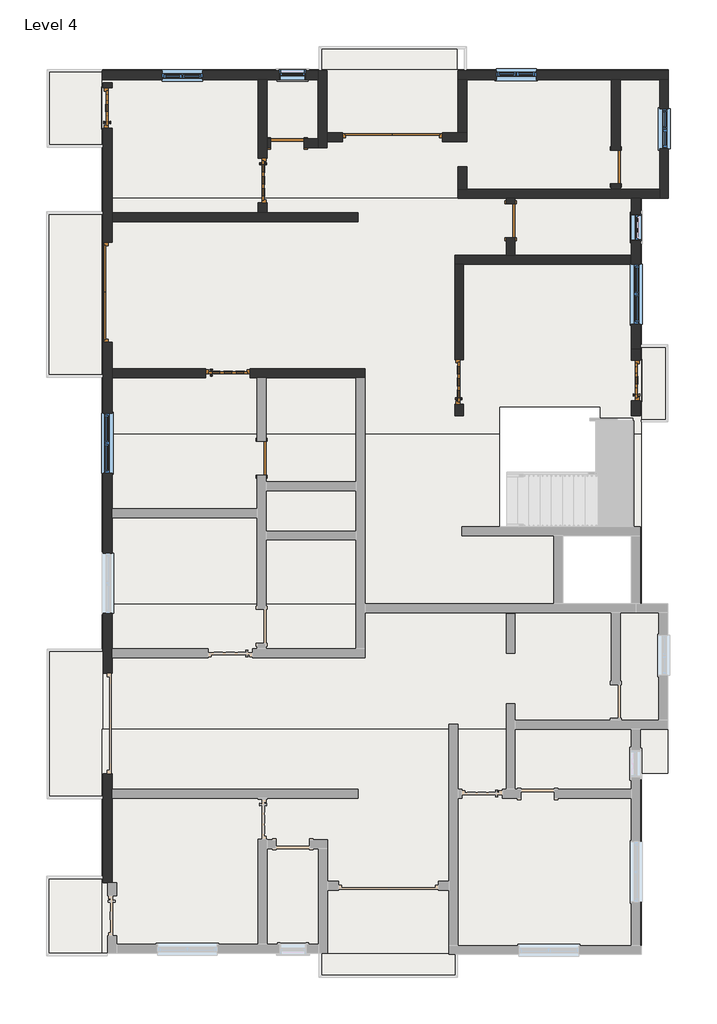
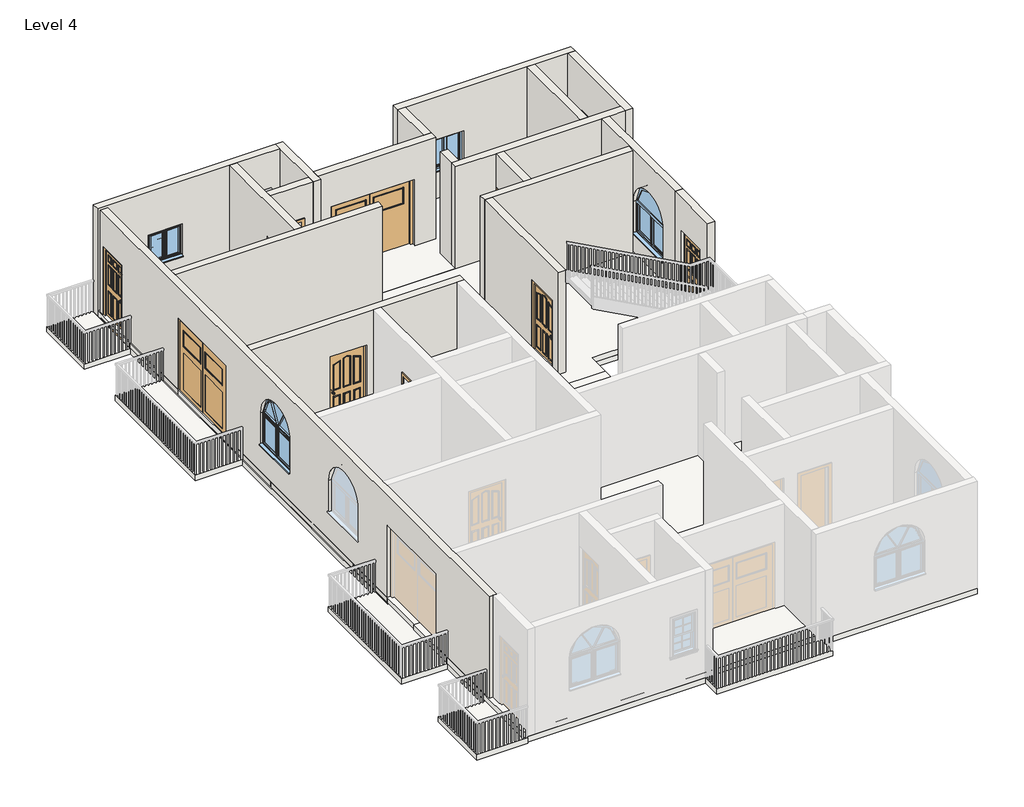
# One storey, part 2 of 7: 19 walls, 11 doors, 10 slabs, 7 windows, 5 roofs.
# Revit data of these elements (continued)
# Type "Windows_Dbl_w-Glazing_Bars : 910x910mm" (continued)
#   Window Board Extension = 0' - 0.98425"
#   Visual Light Transmittance = 0.9
#   Solar Heat Gain Coefficient = 0.78
#   Rough Width = 2' - 11.82677"
#   Rough Height = 2' - 11.82677"
#   Height = 2' - 11.82677"
#   Width = 2' - 11.82677"
#   Heat Transfer Coefficient (U) = 0.6496 BTU/(h·ft²·°F)
#   Glazing Thickness = 0' - 0.94488"
#   Glazing Bar Thickness = 0' - 0.7874"
#   FrameOffset - External = 0' - 1.9685"
#   Frame Depth = 0' - 2.55906"
#   Default Head Height = 6' - 10.67717"
#   Cill Depth = 0' - 3.44488"
#   Cavity Closer Width = 0' - 1.9685"
#   Cavity Closer Offset from Ext = 0' - 4.03543"
#   Cavity Closer Depth = 0' - 3.34646"
#   Vis - Glazing Bars = yes
#   Vis - Cavity Closers = yes
#   Define Thermal Properties by = 1
#   Material Trim = Window Frame
#   Material Glazing Bars = Window Frame
#   Material Glass = Glass
#   Material Frame = Window Frame
#   Wall Closure = (empty or 0)
# Elements 1, 2 (IfcDoor, "Doors_ExtSgl_5 : 910x2110mm")
#   Phase Created = New Construction
#   Materials on its faces: "Door - Panel", "Door - Handle", "Door - Frame/Mullion", "Door - Glazing"
# Elements 3, 4, 5 (IfcDoor, "Doors_ExtSgl_6 : 1010x2110mm")
#   Phase Created = New Construction
#   Materials on its faces: "Door - Panel", "Door - Handle", "Door - Frame/Mullion", "Door - Glazing"
# Element 6 (IfcDoor, "Doors_Garage_Timber_Side_Hung_Glazing : 2270x2050mm")
#   Phase Created = New Construction
#   Materials on its faces: "Door - Panel", "Door - Frame/Mullion", "Door - Glazing"
# Element 7 (IfcDoor, "Doors_Garage_Timber_Side_Hung_Glazing : 2270x2200mm")
#   Phase Created = New Construction
#   Materials on its faces: "Door - Panel", "Door - Frame/Mullion", "Door - Glazing"
# Elements 8, 9, 10, 11 (IfcDoor, "Single-Flush : 30\" x 80\"")
#   Phase Created = New Construction
#   Materials on its faces: "Door - Frame", "Door - Panel"
# Elements 12, 16 (IfcRoof, "Generic - 12\"")
#   built-in parameter 1001705 = 30.5 (stored number, unit not read)
#   built-in parameter 1001710 = 33615
#   Phase Created = New Construction
#   Materials on its faces: "Default Roof", "Earth"
# Elements 13, 15 (IfcRoof, "Generic - 12\"")
#   built-in parameter 1001705 = 30.5 (stored number, unit not read)
#   built-in parameter 1001710 = 33615
#   Phase Created = New Construction
#   Materials on its faces: "Default Roof", "Wood - Stained"
# Element 14 (IfcRoof, "Generic - 12\"")
#   built-in parameter 1001705 = 30.5 (stored number, unit not read)
#   built-in parameter 1001710 = 33615
#   Phase Created = New Construction
#   Materials on its faces: "Default Roof", "Concrete, Lightweight"
# Element 17 (IfcSlab, "Generic - 12\"")
#   Height Offset From Level = 0' - 0"
#   Phase Created = New Construction
#   Materials on its faces: "Default Floor", "Concrete, Lightweight"
# Element 18 (IfcSlab, "Generic - 12\"")
#   Height Offset From Level = 0' - 0"
#   Phase Created = New Construction
#   Materials on its faces: "Default Floor", "Concrete, Lightweight", "Wood - Stained", "Earth"
# Element 19 (IfcSlab, "Generic - 12\"")
#   Height Offset From Level = 0' - 0"
#   Phase Created = New Construction
#   Materials on its faces: "Default Floor", "Earth"
# Element 20 (IfcSlab, "Generic - 12\"")
#   Height Offset From Level = 0' - 0"
#   Phase Created = New Construction
#   Materials on its faces: "Default Floor", "Brick, Soldier Course"
# Elements 21, 22, 23, 24, 25 (IfcSlab, "Generic - 12\"")
#   Height Offset From Level = 0' - 0"
#   Phase Created = New Construction
#   Materials on its faces: "Default Floor"
# Element 26 (IfcSlab, "Generic - 12\"")
#   Height Offset From Level = 0' - 0"
#   Phase Created = New Construction
#   Materials on its faces: "Default Floor", "Earth", "Concrete, Lightweight"
# Elements 27, 31 (IfcWall, "Generic - 9\" w")
#   Top Offset = 0' - 0"
#   Base Offset = 0' - 0"
#   wall height = 10' - 0"
#   Phase Created = New Construction
#   Base Constraint = Level 4
#   Top Constraint = Level 5
#   Materials on its faces: "Default Wall", "Earth"
# Element 28 (IfcWall, "Generic - 9\" w")
#   Top Offset = 0' - 0"
#   Base Offset = 0' - 0"
#   wall height = 10' - 0"
#   Phase Created = New Construction
#   Base Constraint = Level 4
#   Top Constraint = Level 5
#   Materials on its faces: "Default Wall", "Wood - Stained"
# Element 29 (IfcWall, "Generic - 9\" w")
#   Top Offset = 0' - 0"
#   Base Offset = 0' - 0"
#   wall height = 10' - 0"
#   Phase Created = New Construction
#   Base Constraint = Level 4
#   Top Constraint = Level 5
#   Materials on its faces: "Default Wall", "Grass"
# Element 30 (IfcWall, "Generic - 9\" w")
#   Top Offset = 0' - 0"
#   Base Offset = 0' - 0"
#   wall height = 10' - 0"
#   Phase Created = New Construction
#   Base Constraint = Level 4
#   Top Constraint = Level 5
#   Materials on its faces: "Default Wall", "mm"
# Elements 32, 33, 35, 37, 38, 40, 41, 42, 43, 44, 45 (IfcWall, "Generic -4.5\" p")
#   Top Offset = 0' - 0"
#   Base Offset = 0' - 0"
#   wall height = 10' - 0"
#   Phase Created = New Construction
#   Base Constraint = Level 4
#   Top Constraint = Level 5
#   Materials on its faces: "Default Wall"
# Elements 34, 39 (IfcWall, "Generic -4.5\" p")
#   Top Offset = 0' - 0"
#   Base Offset = 0' - 0"
#   wall height = 10' - 0"
#   Phase Created = New Construction
#   Base Constraint = Level 4
#   Top Constraint = Level 5
#   Materials on its faces: "Default Wall", "Earth"
# Element 36 (IfcWall, "Generic -4.5\" p")
#   Top Offset = 0' - 0"
#   Base Offset = 0' - 0"
#   wall height = 10' - 0"
#   Phase Created = New Construction
#   Base Constraint = Level 4
#   Top Constraint = Level 5
#   Materials on its faces: "Default Wall", "Oak Flooring"
# Element 46 (IfcWindow, "Window-Double-Hung : 24\" x 42\"")
#   Mark = "48"
#   Window Inset = 0' - 0"
#   Interior Wall Closure = 0' - 1 1/2"
#   Frame Extension = 0' - 1 1/4"
#   Exterior Wall Closure = 0' - 0 1/2"
#   Interior Trim Visibility = yes
#   Indicator Visibility = yes
#   Exterior Trim Visibility = yes
#   Phase Created = New Construction
#   Materials on its faces: "Wood - Stained", "Glass", "Clad - White"
# Element 47 (IfcWindow, "Window-Double-Hung : 24\" x 42\"")
#   Mark = "54"
#   Window Inset = 0' - 0"
#   Interior Wall Closure = 0' - 1 1/2"
#   Frame Extension = 0' - 1 1/4"
#   Exterior Wall Closure = 0' - 0 1/2"
#   Interior Trim Visibility = yes
#   Indicator Visibility = yes
#   Exterior Trim Visibility = yes
#   Phase Created = New Construction
#   Materials on its faces: "Wood - Stained", "Glass", "Clad - White"
# Element 48 (IfcWindow, "Windows_Arched : 1360x910mm")
#   Mark = "44"
#   Phase Created = New Construction
#   Materials on its faces: "Window Frame", "Glass"
# Element 49 (IfcWindow, "Windows_Arched : 1360x910mm")
#   Mark = "55"
#   Phase Created = New Construction
#   Materials on its faces: "Window Frame", "Glass"
# Element 50 (IfcWindow, "Windows_Dbl_w-Glazing_Bars : 910x910mm")
#   Mark = "51"
#   Phase Created = New Construction
#   Materials on its faces: "Window Frame", "Glass"
# Element 51 (IfcWindow, "Windows_Dbl_w-Glazing_Bars : 910x910mm")
#   Mark = "52"
#   Phase Created = New Construction
#   Materials on its faces: "Window Frame", "Glass"
# Element 52 (IfcWindow, "Windows_Dbl_w-Glazing_Bars : 910x910mm")
#   Mark = "53"
#   Phase Created = New Construction
#   Materials on its faces: "Window Frame", "Glass"
# Materials
#   "Door - Glazing": colour RGB 0 0 255, transparency 0.75
#   "Door - Panel": class "Wood", colour RGB 210 159 95, transparency 0, Cost = 0
#   "Door - Frame/Mullion": class "Wood", colour RGB 212 179 113, transparency 0
#   "Door - Handle": colour RGB 0 0 0, transparency 0
#   "Door - Frame": colour RGB 118 70 51, transparency 0, Cost = 0
#   "Wood - Stained": class "Wood", colour RGB 224 178 126, transparency 0, Cost = 0
#   "Clad - White": class "Wood", colour RGB 242 242 238, transparency 0, Cost = 0
#   "Glass": class "Glass", colour RGB 0 128 192, transparency 0.75, Description = "Soda Lime Glass", Cost = 0
#   "Window Frame": colour RGB 249 249 249, transparency 0
#   "Default Roof": colour RGB 88 101 114, transparency 0, Cost = 0
#   "Earth": class "Generic", colour RGB 97 75 62, transparency 0, Description = "Soil", Cost = 0
#   "Concrete, Lightweight": class "Concrete", colour RGB 142 141 140, transparency 0, Description = "Lightweight concrete", Cost = 0
#   "Default Floor": colour RGB 128 128 128, transparency 0, Cost = 0
#   "Brick, Soldier Course": class "Masonry", colour RGB 170 98 104, transparency 0, Description = "Common brick soldier coursed", Cost = 0
#   "Default Wall": colour RGB 128 128 128, transparency 0, Cost = 0
#   "Grass": class "Generic", colour RGB 104 137 66, transparency 0, Description = "Physical material.", Cost = 0
#   "mm": class "Generic", colour RGB 128 64 0, transparency 0.5, Cost = 0
#   "Oak Flooring": class "Wood", colour RGB 216 169 114, transparency 0, Description = "Quercus Rubra", Cost = 0
